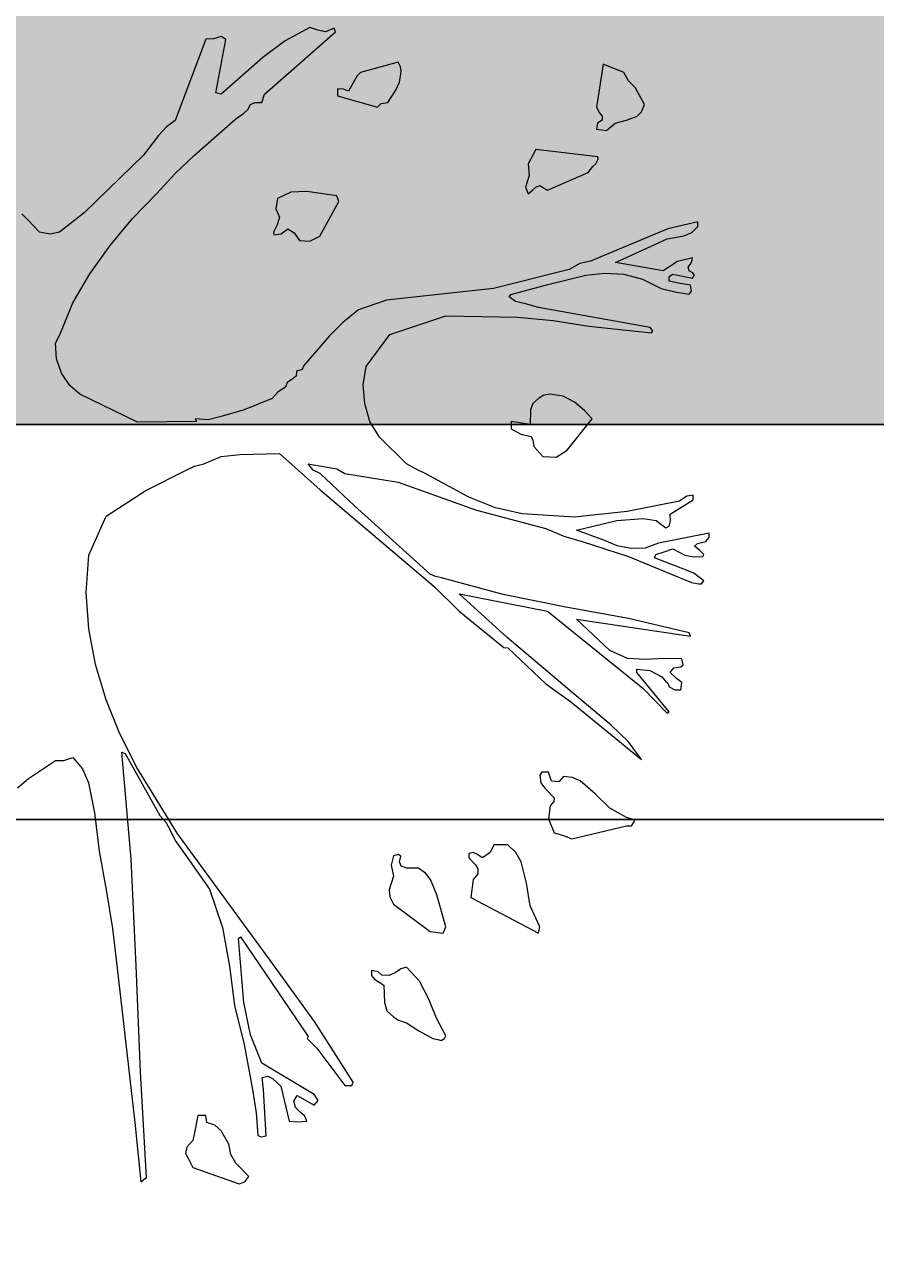
# Model space of a CAD drawing. Units: inches. Extents: x 84 to 1044, y -280 to 906.
# Tile 4 of 105: x 462 to 481, y -132 to -104. Entities that reach past the tile are written whole.
import ezdxf

# ---------------------------------------------------------------- set-up
doc = ezdxf.new("R2010")
doc.units = ezdxf.units.IN
for name, color, linetype, lineweight in [('A-ANNO-DIMS', 2, 'Continuous', 18), ('C-PROP', 7, 'Continuous', 25), ('L-PLNT', 114, 'Continuous', 15)]:
    doc.layers.add(name, color=color, linetype=linetype, lineweight=lineweight)
doc.layers.add('L-PLNT-PATT', color=9, linetype='Continuous', lineweight=9, true_color=0xafd9aa)
doc.styles.get("Standard").update_dxf_attribs({"font": 'arial.ttf'})
doc.dimstyles.get("Standard").update_dxf_attribs({"dimtxt": 0.18, "dimasz": 0.18, "dimexe": 0.18, "dimexo": 0.0625, "dimgap": 0.09, "dimtad": 0, "dimtih": 1, "dimtoh": 1, "dimdec": 4, "dimzin": 0, "dimdsep": 46, "dimtxsty": 'Standard', "dimcen": 0.09, "dimadec": 0, "dimazin": 0, "dimtfac": 1, "dimtdec": 4, "dimtofl": 0, "dimtmove": 0, "dimatfit": 3, "dimfxl": 1, "dimtolj": 1, "dimtzin": 0, "dimarcsym": 0})

# ---------------------------------------------------------------- blocks, each defined once
blk = doc.blocks.new('A$C37E508DF')
for p, q in [((0.3456, 1.093), (0.3469, 1.0964)), ((0.3842, 1.0591), (0.3456, 1.093)), ((0.3469, 1.0964), (0.355, 1.093)), ((0.355, 1.093), (0.3619, 1.0943)), ((0.3619, 1.0943), (0.3692, 1.0968)), ((0.3692, 1.0968), (0.3923, 1.0844)), ((0.4472, 1.0857), (0.4515, 1.0887)), ((0.4515, 1.0887), (0.4584, 1.0865)), ((0.3923, 1.0844), (0.4129, 1.069)), ((0.4562, 1.0364), (0.4472, 1.0857)), ((0.4584, 1.0865), (0.4657, 1.0861)), ((0.4657, 1.0861), (0.4939, 1.0107)), ((0.4129, 1.069), (0.4515, 1.0351)), ((0.0746, 1.0475), (0.0789, 1.0552)), ((0.0789, 1.0552), (0.0978, 1.063)), ((0.0978, 1.063), (0.1042, 1.0231)), ((0.2847, 1.0565), (0.2856, 1.0604)), ((0.2851, 1.054), (0.2847, 1.0565)), ((0.2864, 1.0463), (0.2851, 1.054)), ((0.2856, 1.0604), (0.2877, 1.0647)), ((0.2877, 1.0647), (0.3224, 1.0552)), ((0.3224, 1.0552), (0.3255, 1.0522)), ((0.4112, 1.0351), (0.3842, 1.0591)), ((0.0682, 1.0415), (0.0746, 1.0475)), ((0.2899, 1.039), (0.2864, 1.0463)), ((0.3255, 1.0522), (0.3293, 1.0458)), ((0.3293, 1.0458), (0.3336, 1.0381)), ((0.0596, 1.0257), (0.0682, 1.0415)), ((0.2972, 1.0274), (0.2899, 1.039)), ((0.3439, 1.0338), (0.3066, 1.0231)), ((0.3336, 1.0381), (0.3383, 1.0398)), ((0.3383, 1.0398), (0.3439, 1.0402)), ((0.3439, 1.0402), (0.3439, 1.0338)), ((0.4138, 1.0274), (0.4112, 1.0351)), ((0.4515, 1.0351), (0.4562, 1.0364)), ((0.0626, 1.0188), (0.0596, 1.0257)), ((0.1042, 1.0231), (0.1012, 1.018)), ((0.3032, 1.0265), (0.2972, 1.0274)), ((0.3066, 1.0231), (0.3032, 1.0265)), ((0.4202, 1.0274), (0.4138, 1.0274)), ((0.4241, 1.0257), (0.4202, 1.0274)), ((0.4267, 1.0209), (0.4241, 1.0257)), ((0.4305, 1.0175), (0.4267, 1.0209)), ((0.0665, 1.0149), (0.0626, 1.0188)), ((0.0763, 1.0111), (0.0665, 1.0149)), ((0.087, 1.0085), (0.0763, 1.0111)), ((0.0948, 1.0016), (0.087, 1.0085)), ((0.1012, 1.018), (0.099, 1.0149)), ((0.099, 1.0149), (0.099, 1.0111)), ((0.099, 1.0111), (0.1033, 1.0085)), ((0.1033, 1.0085), (0.1042, 1.0029)), ((0.4378, 1.0124), (0.4305, 1.0175)), ((0.476, 0.9789), (0.4378, 1.0124)), ((0.4939, 1.0107), (0.5021, 1.0051)), ((0.1042, 1.0029), (0.0948, 1.0016)), ((0.5021, 1.0051), (0.5094, 0.9969)), ((0.5094, 0.9969), (0.5231, 0.9789)), ((0.1025, 0.9751), (0.1029, 0.9772)), ((0.1046, 0.9708), (0.1025, 0.9751)), ((0.1029, 0.9772), (0.1604, 0.9841)), ((0.1604, 0.9841), (0.1672, 0.9708)), ((0.4939, 0.9618), (0.476, 0.9789)), ((0.5231, 0.9789), (0.578, 0.9253)), ((0.1076, 0.9682), (0.1046, 0.9708)), ((0.1119, 0.9626), (0.1076, 0.9682)), ((0.1496, 0.9463), (0.1119, 0.9626)), ((0.1672, 0.9708), (0.1664, 0.9601)), ((0.1664, 0.9601), (0.1698, 0.9493)), ((0.5111, 0.9429), (0.4939, 0.9618)), ((0.1565, 0.9506), (0.1496, 0.9463)), ((0.1604, 0.9493), (0.1565, 0.9506)), ((0.1629, 0.9468), (0.1604, 0.9493)), ((0.1672, 0.9429), (0.1629, 0.9468)), ((0.1698, 0.9493), (0.1672, 0.9429)), ((0.3426, 0.936), (0.3443, 0.9412)), ((0.3443, 0.9412), (0.3722, 0.9451)), ((0.3722, 0.9451), (0.3868, 0.9446)), ((0.3868, 0.9446), (0.3992, 0.9386)), ((0.5334, 0.9202), (0.5111, 0.9429)), ((0.3602, 0.9039), (0.3426, 0.936)), ((0.4009, 0.9292), (0.3975, 0.9215)), ((0.3992, 0.9386), (0.4009, 0.9292)), ((0.0103, 0.9129), (0.0103, 0.9172)), ((0.0103, 0.9172), (0.0382, 0.9107)), ((0.3975, 0.9215), (0.3996, 0.9142)), ((0.554, 0.8953), (0.5334, 0.9202)), ((0.578, 0.9253), (0.6011, 0.9077)), ((0.6196, 0.9077), (0.6303, 0.9189)), ((0.6303, 0.9189), (0.6359, 0.9245)), ((0.0159, 0.9073), (0.0103, 0.9129)), ((0.0232, 0.9043), (0.0159, 0.9073)), ((0.0382, 0.9107), (0.1098, 0.8807)), ((0.3838, 0.9069), (0.379, 0.9)), ((0.3898, 0.9107), (0.3838, 0.9069)), ((0.3958, 0.906), (0.3898, 0.9107)), ((0.4026, 0.9052), (0.3958, 0.906)), ((0.3996, 0.9142), (0.4031, 0.9077)), ((0.4031, 0.9077), (0.4026, 0.9052)), ((0.6011, 0.9077), (0.6097, 0.9056)), ((0.6097, 0.9056), (0.6196, 0.9077)), ((0.0386, 0.9013), (0.0232, 0.9043)), ((0.0866, 0.8794), (0.0386, 0.9013)), ((0.3692, 0.8992), (0.3602, 0.9039)), ((0.379, 0.9), (0.3692, 0.8992)), ((0.5728, 0.8691), (0.554, 0.8953)), ((0.0159, 0.8803), (0.0154, 0.8837)), ((0.0154, 0.8837), (0.0292, 0.8803)), ((0.015, 0.87), (0.0184, 0.8717)), ((0.0176, 0.8777), (0.0159, 0.8803)), ((0.0193, 0.8752), (0.0176, 0.8777)), ((0.0184, 0.8717), (0.0193, 0.8752)), ((0.0292, 0.8803), (0.0424, 0.8717)), ((0.0424, 0.8717), (0.0866, 0.8794)), ((0.1098, 0.8807), (0.1196, 0.8786)), ((0.1196, 0.8786), (0.1295, 0.873)), ((0.1295, 0.873), (0.1994, 0.8554)), ((0.0133, 0.8679), (0.015, 0.87)), ((0.0154, 0.8649), (0.0133, 0.8679)), ((0.0334, 0.8687), (0.0154, 0.8649)), ((0.0171, 0.8584), (0.0266, 0.8602)), ((0.0266, 0.8602), (0.0369, 0.8623)), ((0.0369, 0.8666), (0.0334, 0.8687)), ((0.0369, 0.8623), (0.0369, 0.8666)), ((0.0617, 0.864), (0.0442, 0.8554)), ((0.0789, 0.8687), (0.0617, 0.864)), ((0.0965, 0.8696), (0.0789, 0.8687)), ((0.1141, 0.8679), (0.0965, 0.8696)), ((0.1492, 0.8593), (0.1141, 0.8679)), ((0.1835, 0.8499), (0.1492, 0.8593)), ((0.5887, 0.8421), (0.5728, 0.8691)), ((0.0163, 0.8529), (0.0171, 0.8584)), ((0.0184, 0.8503), (0.0163, 0.8529)), ((0.0317, 0.8524), (0.0184, 0.8503)), ((0.0442, 0.8554), (0.0317, 0.8524)), ((0.1848, 0.8477), (0.1835, 0.8499)), ((0.1994, 0.8554), (0.2984, 0.8447)), ((0.0545, 0.8194), (0.1578, 0.8378)), ((0.1578, 0.8378), (0.1698, 0.8413)), ((0.1698, 0.8413), (0.1792, 0.8434)), ((0.1792, 0.8434), (0.1848, 0.8477)), ((0.2984, 0.8447), (0.3242, 0.8357)), ((0.6007, 0.8125), (0.5887, 0.8421)), ((0.1441, 0.8258), (0.1111, 0.8207)), ((0.1771, 0.8288), (0.1441, 0.8258)), ((0.2436, 0.8301), (0.1771, 0.8288)), ((0.2954, 0.813), (0.2436, 0.8301)), ((0.3242, 0.8357), (0.3387, 0.8241)), ((0.0519, 0.8164), (0.0545, 0.8194)), ((0.0532, 0.8143), (0.0519, 0.8164)), ((0.1111, 0.8207), (0.0532, 0.8143)), ((0.3387, 0.8241), (0.3512, 0.8117)), ((0.3173, 0.7834), (0.2954, 0.813)), ((0.3512, 0.8117), (0.3748, 0.7842)), ((0.6046, 0.8048), (0.6007, 0.8125)), ((0.6037, 0.7903), (0.6046, 0.8048)), ((0.3199, 0.7662), (0.3173, 0.7834)), ((0.3748, 0.7842), (0.3765, 0.7804)), ((0.3765, 0.7804), (0.3816, 0.7791)), ((0.3816, 0.7791), (0.382, 0.7744)), ((0.599, 0.777), (0.6037, 0.7903)), ((0.382, 0.7744), (0.3859, 0.7714)), ((0.3859, 0.7714), (0.3902, 0.7684)), ((0.3902, 0.7684), (0.3919, 0.7641)), ((0.5913, 0.7658), (0.599, 0.777)), ((0.1351, 0.7559), (0.1471, 0.7577)), ((0.1471, 0.7577), (0.1527, 0.7568)), ((0.1527, 0.7568), (0.1578, 0.7538)), ((0.3186, 0.7491), (0.3199, 0.7662)), ((0.3919, 0.7641), (0.3988, 0.7598)), ((0.3988, 0.7598), (0.4043, 0.7538)), ((0.5287, 0.7319), (0.5823, 0.7577)), ((0.5823, 0.7577), (0.5913, 0.7658)), ((0.1153, 0.7427), (0.1244, 0.7504)), ((0.1244, 0.7504), (0.1351, 0.7559)), ((0.1578, 0.7538), (0.1629, 0.7491)), ((0.1629, 0.7491), (0.1651, 0.7431)), ((0.3139, 0.7324), (0.3186, 0.7491)), ((0.4043, 0.7538), (0.4301, 0.7431)), ((0.1081, 0.7349), (0.1153, 0.7427)), ((0.1312, 0.7058), (0.1081, 0.7349)), ((0.1651, 0.7431), (0.1655, 0.7298)), ((0.4301, 0.7431), (0.4515, 0.7371)), ((0.4515, 0.7371), (0.4635, 0.7341)), ((0.4635, 0.7341), (0.4755, 0.7349)), ((0.4755, 0.7349), (0.4742, 0.7324)), ((0.1655, 0.7298), (0.1831, 0.7324)), ((0.1831, 0.7255), (0.1741, 0.7208)), ((0.1831, 0.7324), (0.1831, 0.7255)), ((0.3049, 0.7178), (0.3139, 0.7324)), ((0.4742, 0.7324), (0.5287, 0.7319)), ((0.1629, 0.7152), (0.1621, 0.7092)), ((0.1646, 0.7186), (0.1629, 0.7152)), ((0.1741, 0.7208), (0.1646, 0.7186)), ((0.28, 0.6933), (0.3049, 0.7178)), ((0.1415, 0.6994), (0.1312, 0.7058)), ((0.1539, 0.7002), (0.1415, 0.6994)), ((0.1621, 0.7092), (0.1539, 0.7002)), ((0.3975, 0.7028), (0.3598, 0.6693)), ((0.4339, 0.7019), (0.3975, 0.7028)), ((0.4515, 0.7002), (0.4339, 0.7019)), ((0.4674, 0.6933), (0.4515, 0.7002)), ((0.262, 0.6839), (0.271, 0.6882)), ((0.271, 0.6882), (0.28, 0.6933)), ((0.3443, 0.6886), (0.337, 0.6843)), ((0.3533, 0.6903), (0.3443, 0.6886)), ((0.3709, 0.6933), (0.3533, 0.6903)), ((0.3662, 0.6873), (0.3709, 0.6933)), ((0.476, 0.6912), (0.4674, 0.6933)), ((0.4832, 0.6878), (0.476, 0.6912)), ((0.521, 0.6685), (0.4832, 0.6878)), ((0.2877, 0.6762), (0.2152, 0.6505)), ((0.2221, 0.6625), (0.262, 0.6839)), ((0.337, 0.6843), (0.2877, 0.6762)), ((0.328, 0.6543), (0.3598, 0.6843)), ((0.3598, 0.6843), (0.3662, 0.6873)), ((0.3598, 0.6693), (0.2543, 0.5797)), ((0.5578, 0.6449), (0.521, 0.6685)), ((0.0146, 0.6599), (0.0146, 0.6642)), ((0.0146, 0.6642), (0.0206, 0.6633)), ((0.036, 0.6466), (0.0146, 0.6599)), ((0.0206, 0.6633), (0.0274, 0.6586)), ((0.0274, 0.6586), (0.0759, 0.6492)), ((0.1977, 0.6526), (0.2221, 0.6625)), ((0.2581, 0.5913), (0.328, 0.6543)), ((0.0356, 0.6406), (0.036, 0.6466)), ((0.0609, 0.6428), (0.0489, 0.641)), ((0.0853, 0.641), (0.0609, 0.6428)), ((0.0759, 0.6492), (0.1244, 0.644)), ((0.1244, 0.644), (0.1728, 0.647)), ((0.2152, 0.6505), (0.1509, 0.6333)), ((0.1728, 0.647), (0.1977, 0.6526)), ((0.5737, 0.6089), (0.5578, 0.6449)), ((0.0369, 0.6355), (0.0356, 0.6406)), ((0.0399, 0.6342), (0.0369, 0.6355)), ((0.0489, 0.641), (0.0399, 0.6342)), ((0.1226, 0.632), (0.0853, 0.641)), ((0.0973, 0.6226), (0.1226, 0.632)), ((0.1509, 0.6333), (0.1342, 0.6265)), ((0, 0.629), (0.0467, 0.62)), ((0, 0.6252), (0, 0.629)), ((0.003, 0.6213), (0, 0.6252)), ((0.0069, 0.6204), (0.003, 0.6213)), ((0.0107, 0.6196), (0.0069, 0.6204)), ((0.0133, 0.617), (0.0107, 0.6196)), ((0.0467, 0.62), (0.0592, 0.6153)), ((0.1175, 0.6213), (0.0746, 0.6076)), ((0.0849, 0.6175), (0.0973, 0.6226)), ((0.1342, 0.6265), (0.1175, 0.6213)), ((0.0047, 0.6093), (0.0086, 0.6132)), ((0.0056, 0.6076), (0.0047, 0.6093)), ((0.0141, 0.6072), (0.0056, 0.6076)), ((0.0086, 0.6132), (0.0133, 0.617)), ((0.0223, 0.6089), (0.0141, 0.6072)), ((0.0746, 0.6076), (0.0163, 0.5836)), ((0.0334, 0.6145), (0.0223, 0.6089)), ((0.0416, 0.6119), (0.0334, 0.6145)), ((0.0493, 0.6093), (0.0416, 0.6119)), ((0.0506, 0.6063), (0.0493, 0.6093)), ((0.0592, 0.6153), (0.072, 0.6149)), ((0.072, 0.6149), (0.0849, 0.6175)), ((0.5763, 0.5741), (0.5737, 0.6089)), ((0.0141, 0.5921), (0.0257, 0.5969)), ((0.0257, 0.5969), (0.0506, 0.6063)), ((0.0047, 0.5849), (0.0141, 0.5921)), ((0.0069, 0.5823), (0.0047, 0.5849)), ((0.1904, 0.5724), (0.2474, 0.5879)), ((0.2474, 0.5879), (0.253, 0.5892)), ((0.253, 0.5892), (0.2581, 0.5913)), ((0.0099, 0.5823), (0.0069, 0.5823)), ((0.0163, 0.5836), (0.0099, 0.5823)), ((0.2311, 0.5729), (0.1496, 0.557)), ((0.1869, 0.5325), (0.2311, 0.5729)), ((0.2543, 0.5797), (0.2311, 0.557)), ((0.5737, 0.5407), (0.5763, 0.5741)), ((0.1325, 0.5608), (0.1904, 0.5724)), ((0.0184, 0.5368), (0.0746, 0.5501)), ((0.1496, 0.557), (0.0613, 0.4858)), ((0.0746, 0.5501), (0.1325, 0.5608)), ((0.2311, 0.557), (0.1899, 0.5235)), ((0.1226, 0.5497), (0.0171, 0.5338)), ((0.0917, 0.5205), (0.1226, 0.5497)), ((0.5677, 0.5077), (0.5737, 0.5407)), ((0.0171, 0.5338), (0.0184, 0.5368)), ((0.1269, 0.482), (0.1869, 0.5325)), ((0.0755, 0.5133), (0.0917, 0.5205)), ((0.1861, 0.5231), (0.1509, 0.4897)), ((0.1899, 0.5235), (0.1861, 0.5231)), ((0.024, 0.5072), (0.0253, 0.5128)), ((0.0262, 0.5055), (0.024, 0.5072)), ((0.0253, 0.5128), (0.042, 0.5133)), ((0.0326, 0.5047), (0.0262, 0.5055)), ((0.036, 0.5004), (0.0326, 0.5047)), ((0.042, 0.5133), (0.0587, 0.5124)), ((0.0587, 0.5124), (0.0755, 0.5133)), ((0.5578, 0.4751), (0.5677, 0.5077)), ((0.0253, 0.491), (0.03, 0.4948)), ((0.03, 0.4948), (0.036, 0.5004)), ((0.0369, 0.4639), (0.0669, 0.5004)), ((0.0437, 0.4961), (0.0403, 0.4922)), ((0.0549, 0.5021), (0.0437, 0.4961)), ((0.0669, 0.5034), (0.0549, 0.5021)), ((0.0669, 0.5004), (0.0669, 0.5034)), ((0.0262, 0.4841), (0.0253, 0.491)), ((0.0317, 0.4841), (0.0262, 0.4841)), ((0.0369, 0.4871), (0.0317, 0.4841)), ((0.0382, 0.4905), (0.0369, 0.4871)), ((0.0403, 0.4922), (0.0382, 0.4905)), ((0.0613, 0.4858), (0.0386, 0.4627)), ((0.0905, 0.4515), (0.1269, 0.482)), ((0.1509, 0.4897), (0.1282, 0.4734)), ((0.1282, 0.4734), (0.0626, 0.4198)), ((0.545, 0.4434), (0.5578, 0.4751)), ((0.0386, 0.4627), (0.0369, 0.4639)), ((0.0746, 0.4361), (0.0905, 0.4515)), ((0.0626, 0.4198), (0.0746, 0.4361)), ((0.5295, 0.4125), (0.545, 0.4434)), ((0.5403, 0.4254), (0.5081, 0.3679)), ((0.5347, 0.3276), (0.5433, 0.4266)), ((0.5433, 0.4266), (0.5403, 0.4254)), ((0.4922, 0.3516), (0.5295, 0.4125)), ((0.5887, 0.4215), (0.5797, 0.4112)), ((0.5969, 0.4189), (0.5887, 0.4215)), ((0.6046, 0.4189), (0.5969, 0.4189)), ((0.6295, 0.4022), (0.6046, 0.4189)), ((0.1192, 0.4001), (0.1265, 0.4031)), ((0.1265, 0.4031), (0.1346, 0.4039)), ((0.1346, 0.4039), (0.1389, 0.3992)), ((0.1458, 0.3996), (0.1471, 0.4035)), ((0.1471, 0.4035), (0.1484, 0.4082)), ((0.1484, 0.4082), (0.1548, 0.4082)), ((0.1548, 0.4082), (0.1565, 0.4052)), ((0.1565, 0.4052), (0.1556, 0.3983)), ((0.5797, 0.4112), (0.5741, 0.3983)), ((0.6397, 0.3936), (0.6295, 0.4022)), ((0.1055, 0.388), (0.1192, 0.4001)), ((0.1389, 0.3992), (0.1458, 0.3996)), ((0.1518, 0.3932), (0.1432, 0.3842)), ((0.1556, 0.3983), (0.1518, 0.3932)), ((0.5741, 0.3983), (0.5686, 0.3705)), ((0.0917, 0.3748), (0.1055, 0.388)), ((0.1432, 0.3842), (0.1436, 0.3808)), ((0.1436, 0.3808), (0.1471, 0.3769)), ((0.0763, 0.3662), (0.0917, 0.3748)), ((0.1471, 0.3769), (0.1484, 0.3649)), ((0.5081, 0.3679), (0.5025, 0.3619)), ((0.5686, 0.3705), (0.5643, 0.3349)), ((0.069, 0.364), (0.0763, 0.3662)), ((0.069, 0.3627), (0.069, 0.364)), ((0.0716, 0.3585), (0.069, 0.3627)), ((0.0763, 0.3585), (0.0716, 0.3585)), ((0.1269, 0.3464), (0.0763, 0.3585)), ((0.1484, 0.3649), (0.1432, 0.352)), ((0.5025, 0.3619), (0.4982, 0.3537)), ((0.1355, 0.3499), (0.1269, 0.3464)), ((0.1432, 0.352), (0.1355, 0.3499)), ((0.4065, 0.2345), (0.4922, 0.3516)), ((0.4939, 0.3447), (0.4884, 0.337)), ((0.4982, 0.3537), (0.4939, 0.3447)), ((0.1737, 0.325), (0.1788, 0.3336)), ((0.1788, 0.3336), (0.1861, 0.3409)), ((0.1861, 0.3409), (0.199, 0.3409)), ((0.199, 0.3409), (0.2024, 0.3336)), ((0.2024, 0.3336), (0.2097, 0.3289)), ((0.2097, 0.3289), (0.2148, 0.3323)), ((0.2148, 0.3323), (0.2182, 0.3336)), ((0.2182, 0.3336), (0.2221, 0.3327)), ((0.2221, 0.3327), (0.2221, 0.3289)), ((0.4884, 0.337), (0.4622, 0.2997)), ((0.5643, 0.3349), (0.5578, 0.2993)), ((0.1689, 0.3053), (0.1737, 0.325)), ((0.2161, 0.3224), (0.214, 0.3186)), ((0.2221, 0.3289), (0.2161, 0.3224)), ((0.2796, 0.3194), (0.2847, 0.3211)), ((0.2847, 0.3211), (0.2864, 0.325)), ((0.2851, 0.3302), (0.2877, 0.3319)), ((0.2864, 0.325), (0.2851, 0.3302)), ((0.2877, 0.3319), (0.292, 0.3306)), ((0.292, 0.3306), (0.2941, 0.322)), ((0.2941, 0.322), (0.292, 0.3117)), ((0.53, 0.229), (0.5347, 0.3276)), ((0.214, 0.3186), (0.214, 0.3139)), ((0.214, 0.3139), (0.2182, 0.3087)), ((0.2577, 0.3087), (0.2624, 0.3147)), ((0.2624, 0.3147), (0.2689, 0.3194)), ((0.2689, 0.3194), (0.2796, 0.3194)), ((0.292, 0.3117), (0.2959, 0.2993)), ((0.1655, 0.2843), (0.1689, 0.3053)), ((0.2182, 0.3087), (0.2204, 0.292)), ((0.2517, 0.2946), (0.2577, 0.3087)), ((0.2959, 0.2993), (0.2954, 0.2928)), ((0.4622, 0.2997), (0.4502, 0.2645)), ((0.5578, 0.2993), (0.5518, 0.2633)), ((0.2204, 0.292), (0.1578, 0.259)), ((0.2436, 0.265), (0.2517, 0.2946)), ((0.2954, 0.2928), (0.292, 0.286)), ((0.1565, 0.265), (0.1655, 0.2843)), ((0.292, 0.286), (0.2581, 0.2607)), ((0.1578, 0.259), (0.1565, 0.265)), ((0.2461, 0.259), (0.2436, 0.265)), ((0.4502, 0.2645), (0.4438, 0.2285)), ((0.2581, 0.2607), (0.2461, 0.259)), ((0.4335, 0.2556), (0.3709, 0.1634)), ((0.4305, 0.1951), (0.4352, 0.2543)), ((0.4352, 0.2543), (0.4335, 0.2556)), ((0.5518, 0.2633), (0.5475, 0.2268)), ((0.3649, 0.1775), (0.4065, 0.2345)), ((0.268, 0.2148), (0.28, 0.2277)), ((0.28, 0.2277), (0.2851, 0.226)), ((0.2851, 0.226), (0.2903, 0.2225)), ((0.2903, 0.2225), (0.2963, 0.22)), ((0.2963, 0.22), (0.3027, 0.2204)), ((0.3027, 0.2204), (0.3061, 0.2234)), ((0.3061, 0.2234), (0.3122, 0.2247)), ((0.3122, 0.22), (0.3096, 0.2165)), ((0.3122, 0.2247), (0.3122, 0.22)), ((0.4438, 0.2285), (0.4391, 0.1921)), ((0.5261, 0.1308), (0.53, 0.229)), ((0.5475, 0.2268), (0.5313, 0.084)), ((0.2594, 0.1981), (0.268, 0.2148)), ((0.301, 0.211), (0.3002, 0.1951)), ((0.3096, 0.2165), (0.301, 0.211)), ((0.2521, 0.1805), (0.2594, 0.1981)), ((0.3002, 0.1951), (0.298, 0.1874)), ((0.4241, 0.1651), (0.4305, 0.1951)), ((0.298, 0.1874), (0.292, 0.1818)), ((0.4391, 0.1921), (0.4301, 0.1561)), ((0.2436, 0.1642), (0.2521, 0.1805)), ((0.28, 0.1762), (0.2684, 0.1689)), ((0.2873, 0.1788), (0.28, 0.1762)), ((0.292, 0.1818), (0.2873, 0.1788)), ((0.3293, 0.1213), (0.3649, 0.1775)), ((0.2448, 0.1616), (0.2436, 0.1642)), ((0.2478, 0.1599), (0.2448, 0.1616)), ((0.2508, 0.1608), (0.2478, 0.1599)), ((0.2556, 0.1616), (0.2508, 0.1608)), ((0.2684, 0.1689), (0.2556, 0.1616)), ((0.3718, 0.1616), (0.3692, 0.1591)), ((0.3709, 0.1634), (0.3718, 0.1616)), ((0.4138, 0.1389), (0.4241, 0.1651)), ((0.3628, 0.1526), (0.337, 0.1183)), ((0.3692, 0.1591), (0.3628, 0.1526)), ((0.4301, 0.1561), (0.4224, 0.1145)), ((0.3653, 0.1098), (0.4138, 0.1389)), ((0.4082, 0.1269), (0.4039, 0.1248)), ((0.4134, 0.1256), (0.4082, 0.1269)), ((0.5205, 0.033), (0.5261, 0.1308)), ((0.3306, 0.1183), (0.3293, 0.1213)), ((0.337, 0.1183), (0.3306, 0.1183)), ((0.3962, 0.1175), (0.3885, 0.0853)), ((0.4039, 0.1248), (0.3962, 0.1175)), ((0.4121, 0.1145), (0.4134, 0.1256)), ((0.3615, 0.1042), (0.3653, 0.1098)), ((0.3653, 0.0999), (0.3615, 0.1042)), ((0.3812, 0.1089), (0.3653, 0.0999)), ((0.3842, 0.1037), (0.3812, 0.1089)), ((0.3825, 0.0978), (0.3842, 0.1037)), ((0.4099, 0.0716), (0.4121, 0.1145)), ((0.4224, 0.1145), (0.4189, 0.093)), ((0.3739, 0.09), (0.3782, 0.0935)), ((0.3782, 0.0935), (0.3825, 0.0978)), ((0.4189, 0.093), (0.4176, 0.072)), ((0.3722, 0.0853), (0.3739, 0.09)), ((0.3808, 0.0845), (0.3722, 0.0853)), ((0.3885, 0.0853), (0.3808, 0.0845)), ((0.4515, 0.0763), (0.4571, 0.0815)), ((0.4571, 0.0815), (0.4648, 0.084)), ((0.4648, 0.084), (0.4657, 0.0905)), ((0.4657, 0.0905), (0.473, 0.0905)), ((0.473, 0.0905), (0.476, 0.0746)), ((0.5313, 0.084), (0.5257, 0.0291)), ((0.4142, 0.0707), (0.4099, 0.0716)), ((0.4176, 0.072), (0.4142, 0.0707)), ((0.4442, 0.0639), (0.4515, 0.0763)), ((0.476, 0.0746), (0.4777, 0.0673)), ((0.4425, 0.0544), (0.4442, 0.0639)), ((0.4777, 0.0673), (0.4832, 0.0613)), ((0.4832, 0.0613), (0.4845, 0.0553)), ((0.4258, 0.0339), (0.4378, 0.0463)), ((0.4378, 0.0463), (0.4425, 0.0544)), ((0.4811, 0.0493), (0.4777, 0.0424)), ((0.4845, 0.0553), (0.4811, 0.0493)), ((0.4777, 0.0424), (0.4348, 0.0274)), ((0.4296, 0.0291), (0.4258, 0.0339)), ((0.4348, 0.0274), (0.4296, 0.0291)), ((0.5257, 0.0291), (0.5205, 0.033))]:
    blk.add_line(p, q)
blk = doc.blocks.new('*D60')
at = {"layer": 'A-ANNO-DIMS', "color": 0, "lineweight": -2, "transparency": 16777216}
for p, q in [((134.179, -121.942), (134.179, -180.64)), ((992.074, -121.942), (992.074, -180.64)), ((134.359, -180.46), (562.733, -180.46)), ((991.894, -180.46), (563.521, -180.46))]:
    blk.add_line(p, q, dxfattribs=at)
at = {"layer": 'A-ANNO-DIMS', "color": 0, "transparency": 16777216}
for points in [[(134.359, -180.43), (134.359, -180.49), (134.179, -180.46)], [(991.894, -180.43), (991.894, -180.49), (992.074, -180.46)]]:
    blk.add_solid(points, dxfattribs=at)
at = {"layer": 'Defpoints', "color": 0, "transparency": 16777216}
for p in [(134.179, -121.88), (992.074, -121.88), (992.074, -180.46)]:
    blk.add_point(p, dxfattribs=at)
at = {"layer": 'A-ANNO-DIMS', "color": 0, "transparency": 16777216, "insert": (563.127, -180.46), "char_height": 0.18, "attachment_point": 5}
blk.add_mtext('\\A1;857.9', dxfattribs=at)

msp = doc.modelspace()

# ---------------------------------------------------------------- hatches: boundary and pattern name
at = {"layer": 'L-PLNT-PATT', "transparency": 33554597}
h = msp.add_hatch(color=256, dxfattribs=at)
h.dxf.hatch_style = 1
h.paths.add_polyline_path([(504.574, -40.88), (455.074, -40.88), (455.074, -112.88), (504.574, -112.88)])

# ---------------------------------------------------------------- linework, layer by layer
at = {"layer": 'C-PROP'}
for points in [[(504.574, -112.88), (455.074, -112.88)], [(504.574, -121.88), (455.074, -121.88)]]:
    msp.add_lwpolyline(points, dxfattribs=at)

# ---------------------------------------------------------------- block references
at = {"layer": 'L-PLNT', "xscale": -24.64361536662419, "yscale": 24.64361536662419, "zscale": 24.64361536662419}
msp.add_blockref('A$C37E508DF', (477.187, -130.86), dxfattribs=at)

# ---------------------------------------------------------------- dimensions: what is measured, and where the dimension line sits
at = {"layer": 'A-ANNO-DIMS'}
dim = msp.add_linear_dim(base=(992.074, -180.46), p1=(134.179, -121.88), p2=(992.074, -121.88), dimstyle='Standard', override={"dimdec": 1, "dimlfac": 1, "dimrnd": 0, "dimzin": 0, "dimdsep": 46, "dimlunit": 2}, dxfattribs=at)
dim.commit()
dim.dimension.update_dxf_attribs({"geometry": '*D60', "text_midpoint": (563.127, -180.46)})

doc.saveas('drawing.dxf')
